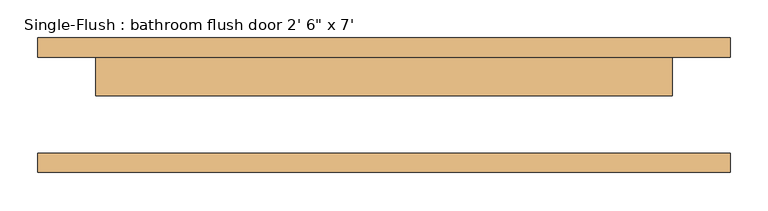
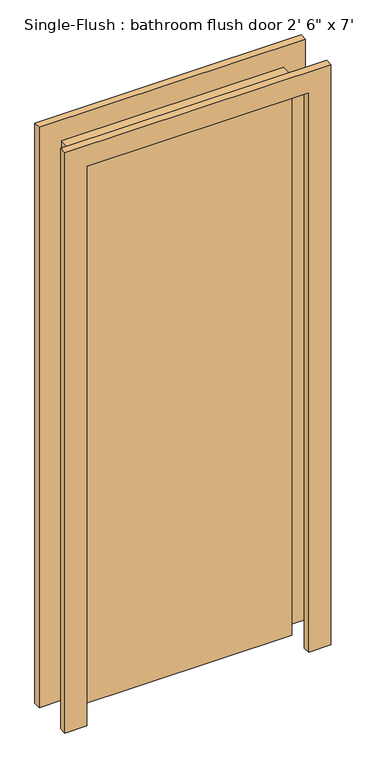
"""IFC4 building model written with IfcOpenShell, lengths in millimetres: door geometry."""

from ifc_helpers import new_model, si_unit, frame, origin, origin_with_axes, place, context, project, spatial, polyline, outline, extrude, source, transform, mapped, element, save


def door_1fe7f57d(model_context):
    return source(origin(), model_context, "Body", "SweptSolid", [
        extrude(outline(polyline([(2108.2, -457.2), (0.0, -457.2), (0.0, -381.0), (2032.0, -381.0), (2032.0, 381.0), (0.0, 381.0), (0.0, 457.2), (2108.2, 457.2), (2108.2, -457.2)])), frame((0.0, 63.5, 0.0), z_axis=(0.0, 1.0, 0.0), x_axis=(0.0, 0.0, 1.0)), (0.0, 0.0, 1.0), 25.4),
        extrude(outline(polyline([(2108.2, 457.2), (2108.2, -457.2), (0.0, -457.2), (0.0, -381.0), (2032.0, -381.0), (2032.0, 381.0), (0.0, 381.0), (0.0, 457.2), (2108.2, 457.2)])), frame((0.0, -88.9, 0.0), z_axis=(0.0, 1.0, 0.0), x_axis=(0.0, 0.0, 1.0)), (0.0, 0.0, 1.0), 25.4),
        extrude(outline(polyline([(381.0, 12.7), (-381.0, 12.7), (-381.0, 63.5), (381.0, 63.5), (381.0, 12.7)])), origin_with_axes(), (0.0, 0.0, 1.0), 2032.0),
    ])


if __name__ == "__main__":
    model = new_model("IFC4")
    model_context = context("Model", 3, world=origin())
    ifc_project = project(units=[si_unit("LENGTHUNIT", "METRE", prefix="MILLI")], contexts=[model_context])
    site = spatial("IfcSite", under=ifc_project)
    building = spatial("IfcBuilding", under=site)
    placement = place(None, origin())
    door_shape = door_1fe7f57d(model_context)
    element("IfcDoor", 1, ObjectType="Single-Flush : bathroom flush door 2' 6\" x 7'", at=placement, inside=building, context=model_context, shape_type="MappedRepresentation", body=[
        mapped(door_shape, transform((0.0, 0.0, 0.0), x_axis=(1.0, 0.0, 0.0), y_axis=(0.0, 1.0, 0.0), z_axis=(0.0, 0.0, 1.0))),
    ])
    save(model, "model.ifc")

# Revit data of these elements
# Type "Single-Flush : bathroom flush door 2' 6\" x 7'"
#   Type Mark = "9"
#   Construction Type Id = "MDOOR"
#   Assembly Code = "C1020"
#   Analytic Construction = "Metal"
#   Thickness = 0' - 2"
#   Heat Transfer Coefficient (U) = 0.651978 BTU/(h·ft²·°F)
#   Height = 6' - 8"
#   Trim Projection Ext = 0' - 1"
#   Trim Projection Int = 0' - 1"
#   Trim Width = 0' - 3"
#   Width = 2' - 6"
#   Define Thermal Properties by = 1
#   Door Material = Door - Panel
#   Frame Material = Door - Frame
#   Visual Light Transmittance = 0
#   Solar Heat Gain Coefficient = 0
#   Function = (empty or 0)
#   Wall Closure = (empty or 0)
# Element 1 (IfcDoor, "Single-Flush : bathroom flush door 2' 6\" x 7'")
#   Materials on its faces: "Door - Frame", "Door - Panel"
# Materials
#   "Door - Panel": class "Wood", colour RGB 210 159 95, transparency 0, Cost = 0
#   "Door - Frame": colour RGB 118 70 51, transparency 0, Cost = 0
